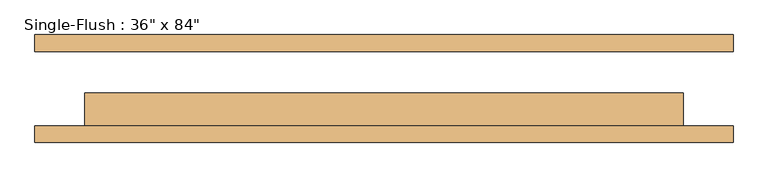
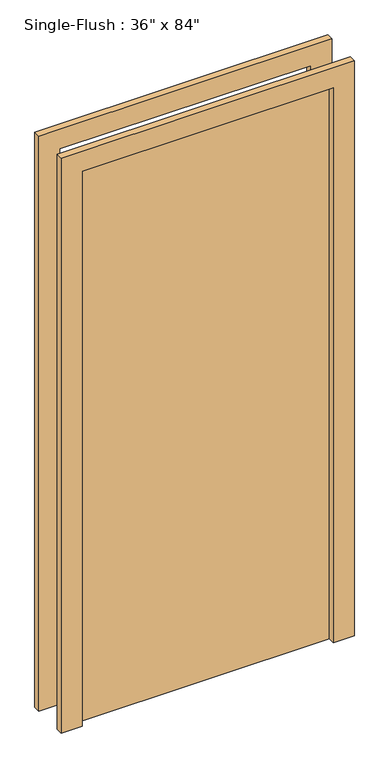
"""IFC4 building model written with IfcOpenShell, lengths in millimetres: door geometry."""

from ifc_helpers import new_model, si_unit, frame, origin, origin_with_axes, place, context, project, spatial, polyline, outline, extrude, source, transform, mapped, element, save


def door_305aa2a5(model_context):
    return source(origin(), model_context, "Body", "SweptSolid", [
        extrude(outline(polyline([(2209.8, -533.4), (0.0, -533.4), (0.0, -457.2), (2133.6, -457.2), (2133.6, 457.2), (0.0, 457.2), (0.0, 533.4), (2209.8, 533.4), (2209.8, -533.4)])), frame((0.0, -82.55, 0.0), z_axis=(0.0, 1.0, 0.0), x_axis=(0.0, 0.0, 1.0)), (0.0, 0.0, 1.0), 25.4),
        extrude(outline(polyline([(2209.8, 533.4), (2209.8, -533.4), (0.0, -533.4), (0.0, -457.2), (2133.6, -457.2), (2133.6, 457.2), (0.0, 457.2), (0.0, 533.4), (2209.8, 533.4)])), frame((0.0, 57.15, 0.0), z_axis=(0.0, 1.0, 0.0), x_axis=(0.0, 0.0, 1.0)), (0.0, 0.0, 1.0), 25.4),
        extrude(outline(polyline([(457.2, -6.35), (457.2, -57.15), (-457.2, -57.15), (-457.2, -6.35), (457.2, -6.35)])), origin_with_axes(), (0.0, 0.0, 1.0), 2133.6),
    ])


if __name__ == "__main__":
    model = new_model("IFC4")
    model_context = context("Model", 3, world=origin())
    ifc_project = project(units=[si_unit("LENGTHUNIT", "METRE", prefix="MILLI")], contexts=[model_context])
    site = spatial("IfcSite", under=ifc_project)
    building = spatial("IfcBuilding", under=site)
    placement = place(None, origin())
    door_shape = door_305aa2a5(model_context)
    element("IfcDoor", 1, ObjectType="Single-Flush : 36\" x 84\"", at=placement, inside=building, context=model_context, shape_type="MappedRepresentation", body=[
        mapped(door_shape, transform((0.0, 0.0, 0.0), x_axis=(1.0, 0.0, 0.0), y_axis=(0.0, 1.0, 0.0), z_axis=(0.0, 0.0, 1.0))),
    ])
    save(model, "model.ifc")

# Revit data of these elements
# Type "Single-Flush : 36\" x 84\""
#   Type Mark = "1"
#   Construction Type Id = "MDOOR"
#   Assembly Code = "C1020"
#   Analytic Construction = "Metal"
#   Thickness = 0' - 2"
#   Heat Transfer Coefficient (U) = 0.651978 BTU/(h·ft²·°F)
#   Height = 7' - 0"
#   Trim Projection Ext = 0' - 1"
#   Trim Projection Int = 0' - 1"
#   Trim Width = 0' - 3"
#   Width = 3' - 0"
#   Define Thermal Properties by = 1
#   Define Thermal Properties by = 1
#   Door Material = Door - Panel
#   Frame Material = Door - Frame
#   Visual Light Transmittance = 0
#   Solar Heat Gain Coefficient = 0
#   Function = (empty or 0)
#   Wall Closure = (empty or 0)
# Element 1 (IfcDoor, "Single-Flush : 36\" x 84\"")
#   Materials on its faces: "Door - Frame", "Door - Panel"
# Materials
#   "Door - Panel": class "Wood", colour RGB 210 159 95, transparency 0, Cost = 0
#   "Door - Frame": colour RGB 118 70 51, transparency 0, Cost = 0
